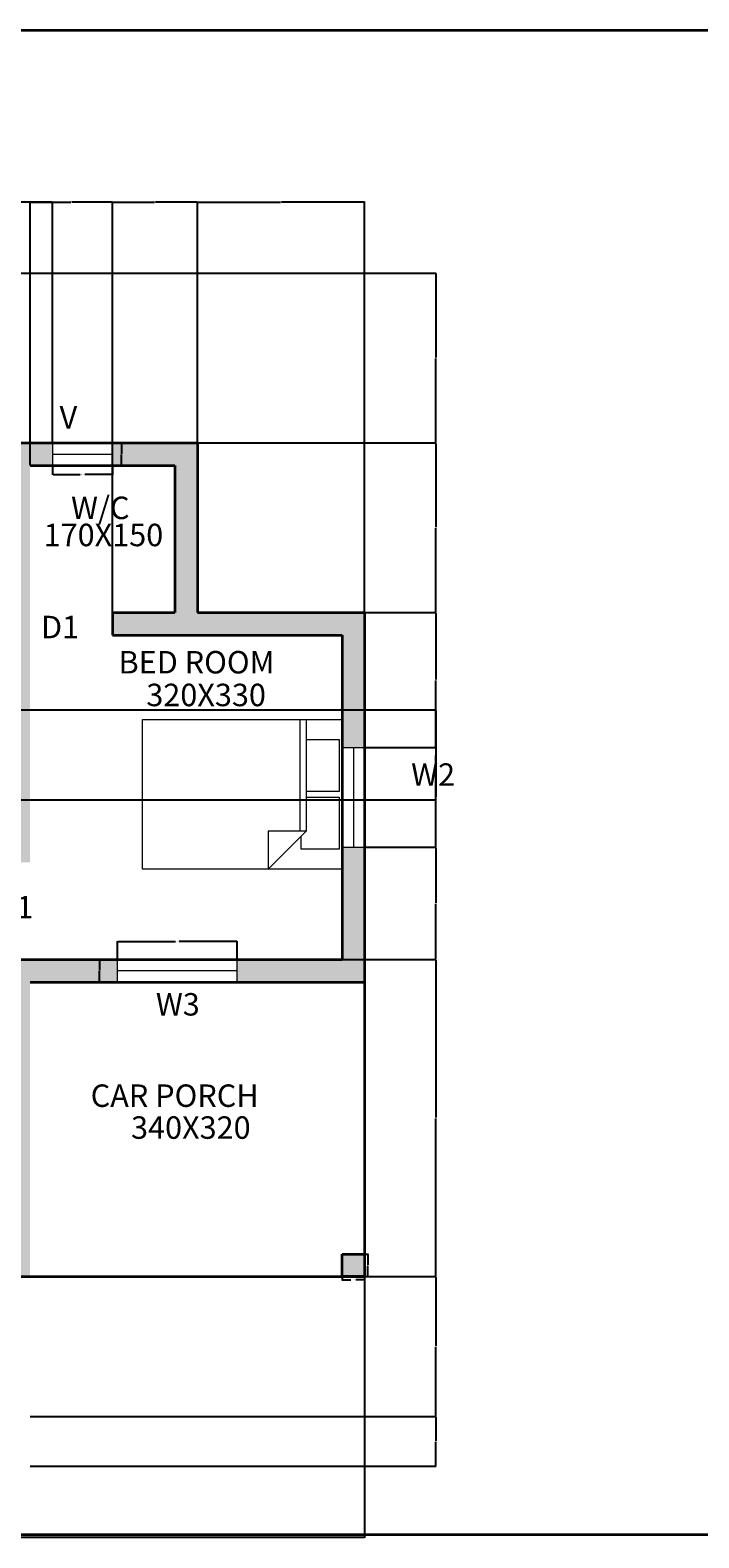
# Model space of a CAD drawing. Units: inches. Extents: x 1332 to 3175, y 1481 to 2088.
# Tile 4 of 5: x 1717 to 1985, y 1484 to 2088. Entities that reach past the tile are written whole.
import ezdxf

# ---------------------------------------------------------------- set-up
doc = ezdxf.new("R2010")
doc.units = ezdxf.units.IN
for name, color, linetype, lineweight in [('A-ANNO-DIMS', 2, 'Continuous', 18), ('A-ANNO-TEXT', 7, 'Continuous', 18), ('A-ANNO-TTLB', 7, 'Continuous', 35), ('A-AREA-IDEN', 7, 'Continuous', 18), ('A-FURN', 8, 'Continuous', 18), ('A-WALL', 7, 'Continuous', 35)]:
    doc.layers.add(name, color=color, linetype=linetype, lineweight=lineweight)
for name, color, linetype, lineweight, true_color in [('A-COLS', 18, 'Continuous', 35, 0x000000), ('A-GLAZ', 30, 'Continuous', 18, 0xf8991e), ('A-WALL-PATT', 18, 'Continuous', 13, 0x000000)]:
    doc.layers.add(name, color=color, linetype=linetype, lineweight=lineweight, true_color=true_color)
doc.styles.get("Standard").update_dxf_attribs({"font": 'arial.ttf'})
doc.dimstyles.get("Standard").update_dxf_attribs({"dimtxt": 0.18, "dimasz": 0.18, "dimexe": 0.18, "dimexo": 0.0625, "dimgap": 0.09, "dimtad": 0, "dimtih": 1, "dimtoh": 1, "dimdec": 4, "dimzin": 0, "dimdsep": 46, "dimtxsty": 'Standard', "dimcen": 0.09, "dimadec": 0, "dimazin": 0, "dimtfac": 1, "dimtdec": 4, "dimtofl": 0, "dimtmove": 0, "dimatfit": 3, "dimfxl": 1, "dimtolj": 1, "dimtzin": 0, "dimarcsym": 0})

# ---------------------------------------------------------------- blocks, each defined once
blk = doc.blocks.new('Bed - Queen')
for p, q in [((0, -80.00003), (0, 0)), ((0, 0), (59.99999, 0)), ((59.99999, 0), (59.99999, -80.00003)), ((7.99999, -1.2), (28.79998, -1.2)), ((7.99999, -14.4), (7.99999, -1.2)), ((28.79998, -1.2), (28.79998, -14.4)), ((31.19999, -1.2), (51.99999, -1.2)), ((31.19999, -14.4), (31.19999, -1.2)), ((51.99999, -1.2), (51.99999, -16.4)), ((0, -14.4), (44.8, -14.4)), ((44.8, -16.8), (0, -16.8)), ((59.99999, -29.6), (44.8, -14.4)), ((44.8, -14.4), (44.8, -29.6)), ((51.99999, -16.4), (46.79936, -16.4)), ((44.8, -29.6), (59.99999, -29.6)), ((59.99999, -80.00003), (0, -80.00003))]:
    blk.add_line(p, q)
blk = doc.blocks.new('COL-SQUARE-9-PLAN')
h = blk.add_hatch(color=256)
h.dxf.hatch_style = 1
h.paths.add_polyline_path([(9, 9), (0, 9), (0, 0), (9, 0)])
blk.add_lwpolyline([(0, 9), (9, 9), (9, 0), (0, 0)], close=True)
blk = doc.blocks.new('WIN-W3-48')
for p, q in [((0, 9), (0, 0)), ((48, 9), (48, 0)), ((0, 4.5), (48, 4.5))]:
    blk.add_line(p, q)
blk = doc.blocks.new('VENT-24')
for p, q in [((0, 9), (0, 0)), ((24, 9), (24, 0)), ((0, 4.5), (24, 4.5))]:
    blk.add_line(p, q)
blk = doc.blocks.new('*D15')
at = {"layer": 'A-ANNO-DIMS', "color": 0, "lineweight": -2, "transparency": 16777216}
for p, q in [((1752.13, 1716.18), (1752.13, 1723.5)), ((1752.31, 1723.32), (1775.38, 1723.32)), ((1799.95, 1723.32), (1776.89, 1723.32)), ((1800.13, 1716.18), (1800.13, 1723.5))]:
    blk.add_line(p, q, dxfattribs=at)
at = {"layer": 'A-ANNO-DIMS', "color": 0, "transparency": 16777216}
for points in [[(1752.31, 1723.35), (1752.31, 1723.29), (1752.13, 1723.32)], [(1799.95, 1723.35), (1799.95, 1723.29), (1800.13, 1723.32)]]:
    blk.add_solid(points, dxfattribs=at)
at = {"layer": 'Defpoints', "color": 0, "transparency": 16777216}
for p in [(1752.13, 1723.32), (1752.13, 1716.12), (1800.13, 1716.12)]:
    blk.add_point(p, dxfattribs=at)
at = {"layer": 'A-ANNO-DIMS', "color": 0, "transparency": 16777216, "insert": (1776.13, 1723.32), "char_height": 0.18, "attachment_point": 5}
blk.add_mtext('\\A1;W3 48 TYP.', dxfattribs=at)
blk = doc.blocks.new('*D16')
at = {"layer": 'A-ANNO-DIMS', "color": 0, "lineweight": -2, "transparency": 16777216}
for p, q in [((1752.07, 1716.12), (1744.75, 1716.12)), ((1744.93, 1715.94), (1744.93, 1711.8)), ((1744.93, 1707.3), (1744.93, 1711.44)), ((1752.07, 1707.12), (1744.75, 1707.12))]:
    blk.add_line(p, q, dxfattribs=at)
at = {"layer": 'A-ANNO-DIMS', "color": 0, "transparency": 16777216}
for points in [[(1744.9, 1715.94), (1744.96, 1715.94), (1744.93, 1716.12)], [(1744.9, 1707.3), (1744.96, 1707.3), (1744.93, 1707.12)]]:
    blk.add_solid(points, dxfattribs=at)
at = {"layer": 'Defpoints', "color": 0, "transparency": 16777216}
for p in [(1752.13, 1716.12), (1744.93, 1707.12), (1752.13, 1707.12)]:
    blk.add_point(p, dxfattribs=at)
at = {"layer": 'A-ANNO-DIMS', "color": 0, "transparency": 16777216, "insert": (1744.93, 1711.62), "char_height": 0.18, "attachment_point": 5}
blk.add_mtext('\\A1;9 TYP.', dxfattribs=at)
blk = doc.blocks.new('*D17')
at = {"layer": 'A-ANNO-DIMS', "color": 0, "lineweight": -2, "transparency": 16777216}
for p, q in [((1726.13, 1914.06), (1726.13, 1910.34)), ((1726.31, 1910.52), (1737.23, 1910.52)), ((1749.95, 1910.52), (1739.03, 1910.52)), ((1750.13, 1914.06), (1750.13, 1910.34))]:
    blk.add_line(p, q, dxfattribs=at)
at = {"layer": 'A-ANNO-DIMS', "color": 0, "transparency": 16777216}
for points in [[(1726.31, 1910.55), (1726.31, 1910.49), (1726.13, 1910.52)], [(1749.95, 1910.55), (1749.95, 1910.49), (1750.13, 1910.52)]]:
    blk.add_solid(points, dxfattribs=at)
at = {"layer": 'Defpoints', "color": 0, "transparency": 16777216}
for p in [(1726.13, 1914.12), (1750.13, 1914.12), (1750.13, 1910.52)]:
    blk.add_point(p, dxfattribs=at)
at = {"layer": 'A-ANNO-DIMS', "color": 0, "transparency": 16777216, "insert": (1738.13, 1910.52), "char_height": 0.18, "attachment_point": 5}
blk.add_mtext('\\A1;VENT 24 TYP.', dxfattribs=at)
blk = doc.blocks.new('*D18')
at = {"layer": 'A-ANNO-DIMS', "color": 0, "lineweight": -2, "transparency": 16777216}
for p, q in [((1750.19, 1923.12), (1753.91, 1923.12)), ((1753.73, 1922.94), (1753.73, 1918.8)), ((1753.73, 1914.3), (1753.73, 1918.44)), ((1750.19, 1914.12), (1753.91, 1914.12))]:
    blk.add_line(p, q, dxfattribs=at)
at = {"layer": 'A-ANNO-DIMS', "color": 0, "transparency": 16777216}
for points in [[(1753.7, 1922.94), (1753.76, 1922.94), (1753.73, 1923.12)], [(1753.7, 1914.3), (1753.76, 1914.3), (1753.73, 1914.12)]]:
    blk.add_solid(points, dxfattribs=at)
at = {"layer": 'Defpoints', "color": 0, "transparency": 16777216}
for p in [(1750.13, 1923.12), (1753.73, 1923.12), (1750.13, 1914.12)]:
    blk.add_point(p, dxfattribs=at)
at = {"layer": 'A-ANNO-DIMS', "color": 0, "transparency": 16777216, "insert": (1753.73, 1918.62), "char_height": 0.18, "attachment_point": 5}
blk.add_mtext('\\A1;9 TYP.', dxfattribs=at)
blk = doc.blocks.new('*D23')
at = {"layer": 'A-ANNO-DIMS', "color": 0, "lineweight": -2, "transparency": 16777216}
for p, q in [((1842.13, 1589.06), (1842.13, 1587.59)), ((1851.13, 1589.06), (1851.13, 1587.59)), ((1842.31, 1587.77), (1845.59, 1587.77)), ((1850.95, 1587.77), (1847.67, 1587.77))]:
    blk.add_line(p, q, dxfattribs=at)
at = {"layer": 'A-ANNO-DIMS', "color": 0, "transparency": 16777216}
for points in [[(1842.31, 1587.8), (1842.31, 1587.74), (1842.13, 1587.77)], [(1850.95, 1587.8), (1850.95, 1587.74), (1851.13, 1587.77)]]:
    blk.add_solid(points, dxfattribs=at)
at = {"layer": 'Defpoints', "color": 0, "transparency": 16777216}
for p in [(1842.13, 1589.12), (1851.13, 1589.12), (1851.13, 1587.77)]:
    blk.add_point(p, dxfattribs=at)
at = {"layer": 'A-ANNO-DIMS', "color": 0, "transparency": 16777216, "insert": (1846.63, 1587.77), "char_height": 0.18, "attachment_point": 5}
blk.add_mtext('\\A1;COLUMN 9 TYP.', dxfattribs=at)
blk = doc.blocks.new('*D24')
at = {"layer": 'A-ANNO-DIMS', "color": 0, "lineweight": -2, "transparency": 16777216}
for p, q in [((1851.19, 1598.12), (1852.66, 1598.12)), ((1852.48, 1597.94), (1852.48, 1593.8)), ((1851.19, 1589.12), (1852.66, 1589.12)), ((1852.48, 1589.3), (1852.48, 1593.44))]:
    blk.add_line(p, q, dxfattribs=at)
at = {"layer": 'A-ANNO-DIMS', "color": 0, "transparency": 16777216}
for points in [[(1852.45, 1597.94), (1852.51, 1597.94), (1852.48, 1598.12)], [(1852.45, 1589.3), (1852.51, 1589.3), (1852.48, 1589.12)]]:
    blk.add_solid(points, dxfattribs=at)
at = {"layer": 'Defpoints', "color": 0, "transparency": 16777216}
for p in [(1851.13, 1598.12), (1852.48, 1598.12), (1851.13, 1589.12)]:
    blk.add_point(p, dxfattribs=at)
at = {"layer": 'A-ANNO-DIMS', "color": 0, "transparency": 16777216, "insert": (1852.48, 1593.62), "char_height": 0.18, "attachment_point": 5}
blk.add_mtext('\\A1;9 TYP.', dxfattribs=at)
blk = doc.blocks.new('*D37')
at = {"layer": 'A-ANNO-DIMS', "color": 0, "lineweight": -2, "transparency": 16777216}
for p, q in [((1851.13, 1589.06), (1851.13, 1484.44)), ((1389.63, 1533.06), (1389.63, 1484.44)), ((1389.81, 1484.62), (1619.98, 1484.62)), ((1850.95, 1484.62), (1620.78, 1484.62))]:
    blk.add_line(p, q, dxfattribs=at)
at = {"layer": 'A-ANNO-DIMS', "color": 0, "transparency": 16777216}
for points in [[(1389.81, 1484.65), (1389.81, 1484.59), (1389.63, 1484.62)], [(1850.95, 1484.65), (1850.95, 1484.59), (1851.13, 1484.62)]]:
    blk.add_solid(points, dxfattribs=at)
at = {"layer": 'Defpoints', "color": 0, "transparency": 16777216}
for p in [(1851.13, 1589.12), (1389.63, 1533.12), (1851.13, 1484.62)]:
    blk.add_point(p, dxfattribs=at)
at = {"layer": 'A-ANNO-DIMS', "color": 0, "transparency": 16777216, "insert": (1620.38, 1484.62), "char_height": 0.18, "attachment_point": 5}
blk.add_mtext('\\A1;461.5', dxfattribs=at)
blk = doc.blocks.new('*D45')
at = {"layer": 'A-ANNO-DIMS', "color": 0, "lineweight": -2, "transparency": 16777216}
for p, q in [((1673.13, 1923.18), (1673.13, 2019.8)), ((1673.31, 2019.62), (1699.41, 2019.62)), ((1725.95, 2019.62), (1699.85, 2019.62)), ((1726.13, 1923.18), (1726.13, 2019.8))]:
    blk.add_line(p, q, dxfattribs=at)
at = {"layer": 'A-ANNO-DIMS', "color": 0, "transparency": 16777216}
for points in [[(1673.31, 2019.65), (1673.31, 2019.59), (1673.13, 2019.62)], [(1725.95, 2019.65), (1725.95, 2019.59), (1726.13, 2019.62)]]:
    blk.add_solid(points, dxfattribs=at)
at = {"layer": 'Defpoints', "color": 0, "transparency": 16777216}
for p in [(1726.13, 2019.62), (1673.13, 1923.12), (1726.13, 1923.12)]:
    blk.add_point(p, dxfattribs=at)
at = {"layer": 'A-ANNO-DIMS', "color": 0, "transparency": 16777216, "insert": (1699.63, 2019.62), "char_height": 0.18, "attachment_point": 5}
blk.add_mtext('\\A1;53', dxfattribs=at)
blk = doc.blocks.new('*D46')
at = {"layer": 'A-ANNO-DIMS', "color": 0, "lineweight": -2, "transparency": 16777216}
for p, q in [((1750.13, 1923.18), (1750.13, 2019.8)), ((1750.31, 2019.62), (1766.91, 2019.62)), ((1783.95, 2019.62), (1767.35, 2019.62)), ((1784.13, 1923.18), (1784.13, 2019.8))]:
    blk.add_line(p, q, dxfattribs=at)
at = {"layer": 'A-ANNO-DIMS', "color": 0, "transparency": 16777216}
for points in [[(1750.31, 2019.65), (1750.31, 2019.59), (1750.13, 2019.62)], [(1783.95, 2019.65), (1783.95, 2019.59), (1784.13, 2019.62)]]:
    blk.add_solid(points, dxfattribs=at)
at = {"layer": 'Defpoints', "color": 0, "transparency": 16777216}
for p in [(1784.13, 2019.62), (1750.13, 1923.12), (1784.13, 1923.12)]:
    blk.add_point(p, dxfattribs=at)
at = {"layer": 'A-ANNO-DIMS', "color": 0, "transparency": 16777216, "insert": (1767.13, 2019.62), "char_height": 0.18, "attachment_point": 5}
blk.add_mtext('\\A1;34', dxfattribs=at)
blk = doc.blocks.new('*D47')
at = {"layer": 'A-ANNO-DIMS', "color": 0, "lineweight": -2, "transparency": 16777216}
for p, q in [((1784.13, 1923.18), (1784.13, 2019.8)), ((1784.31, 2019.62), (1817.41, 2019.62)), ((1850.95, 2019.62), (1817.85, 2019.62)), ((1851.13, 1855.18), (1851.13, 2019.8))]:
    blk.add_line(p, q, dxfattribs=at)
at = {"layer": 'A-ANNO-DIMS', "color": 0, "transparency": 16777216}
for points in [[(1784.31, 2019.65), (1784.31, 2019.59), (1784.13, 2019.62)], [(1850.95, 2019.65), (1850.95, 2019.59), (1851.13, 2019.62)]]:
    blk.add_solid(points, dxfattribs=at)
at = {"layer": 'Defpoints', "color": 0, "transparency": 16777216}
for p in [(1851.13, 2019.62), (1784.13, 1923.12), (1851.13, 1855.12)]:
    blk.add_point(p, dxfattribs=at)
at = {"layer": 'A-ANNO-DIMS', "color": 0, "transparency": 16777216, "insert": (1817.63, 2019.62), "char_height": 0.18, "attachment_point": 5}
blk.add_mtext('\\A1;67', dxfattribs=at)
blk = doc.blocks.new('*D48')
at = {"layer": 'A-ANNO-DIMS', "color": 0, "lineweight": -2, "transparency": 16777216}
for p, q in [((1717.19, 1533.12), (1879.81, 1533.12)), ((1879.63, 1532.94), (1879.63, 1523.3)), ((1879.63, 1513.3), (1879.63, 1522.94)), ((1717.19, 1513.12), (1879.81, 1513.12))]:
    blk.add_line(p, q, dxfattribs=at)
at = {"layer": 'A-ANNO-DIMS', "color": 0, "transparency": 16777216}
for points in [[(1879.6, 1532.94), (1879.66, 1532.94), (1879.63, 1533.12)], [(1879.6, 1513.3), (1879.66, 1513.3), (1879.63, 1513.12)]]:
    blk.add_solid(points, dxfattribs=at)
at = {"layer": 'Defpoints', "color": 0, "transparency": 16777216}
for p in [(1717.13, 1533.12), (1879.63, 1533.12), (1717.13, 1513.12)]:
    blk.add_point(p, dxfattribs=at)
at = {"layer": 'A-ANNO-DIMS', "color": 0, "transparency": 16777216, "insert": (1879.63, 1523.12), "char_height": 0.18, "attachment_point": 5}
blk.add_mtext('\\A1;20', dxfattribs=at)
blk = doc.blocks.new('*D49')
at = {"layer": 'A-ANNO-DIMS', "color": 0, "lineweight": -2, "transparency": 16777216}
for p, q in [((1851.19, 1589.12), (1879.81, 1589.12)), ((1879.63, 1588.94), (1879.63, 1561.3)), ((1879.63, 1533.3), (1879.63, 1560.94)), ((1717.19, 1533.12), (1879.81, 1533.12))]:
    blk.add_line(p, q, dxfattribs=at)
at = {"layer": 'A-ANNO-DIMS', "color": 0, "transparency": 16777216}
for points in [[(1879.6, 1588.94), (1879.66, 1588.94), (1879.63, 1589.12)], [(1879.6, 1533.3), (1879.66, 1533.3), (1879.63, 1533.12)]]:
    blk.add_solid(points, dxfattribs=at)
at = {"layer": 'Defpoints', "color": 0, "transparency": 16777216}
for p in [(1851.13, 1589.12), (1879.63, 1589.12), (1717.13, 1533.12)]:
    blk.add_point(p, dxfattribs=at)
at = {"layer": 'A-ANNO-DIMS', "color": 0, "transparency": 16777216, "insert": (1879.63, 1561.12), "char_height": 0.18, "attachment_point": 5}
blk.add_mtext('\\A1;56', dxfattribs=at)
blk = doc.blocks.new('*D50')
at = {"layer": 'A-ANNO-DIMS', "color": 0, "lineweight": -2, "transparency": 16777216}
for p, q in [((1842.19, 1716.12), (1879.81, 1716.12)), ((1879.63, 1715.94), (1879.63, 1652.8)), ((1879.63, 1589.3), (1879.63, 1652.44)), ((1851.19, 1589.12), (1879.81, 1589.12))]:
    blk.add_line(p, q, dxfattribs=at)
at = {"layer": 'A-ANNO-DIMS', "color": 0, "transparency": 16777216}
for points in [[(1879.6, 1715.94), (1879.66, 1715.94), (1879.63, 1716.12)], [(1879.6, 1589.3), (1879.66, 1589.3), (1879.63, 1589.12)]]:
    blk.add_solid(points, dxfattribs=at)
at = {"layer": 'Defpoints', "color": 0, "transparency": 16777216}
for p in [(1842.13, 1716.12), (1879.63, 1716.12), (1851.13, 1589.12)]:
    blk.add_point(p, dxfattribs=at)
at = {"layer": 'A-ANNO-DIMS', "color": 0, "transparency": 16777216, "insert": (1879.63, 1652.62), "char_height": 0.18, "attachment_point": 5}
blk.add_mtext('\\A1;127', dxfattribs=at)
blk = doc.blocks.new('*D51')
at = {"layer": 'A-ANNO-DIMS', "color": 0, "lineweight": -2, "transparency": 16777216}
for p, q in [((1851.19, 1761.12), (1879.81, 1761.12)), ((1879.63, 1760.94), (1879.63, 1738.8)), ((1879.63, 1716.3), (1879.63, 1738.44)), ((1842.19, 1716.12), (1879.81, 1716.12))]:
    blk.add_line(p, q, dxfattribs=at)
at = {"layer": 'A-ANNO-DIMS', "color": 0, "transparency": 16777216}
for points in [[(1879.6, 1760.94), (1879.66, 1760.94), (1879.63, 1761.12)], [(1879.6, 1716.3), (1879.66, 1716.3), (1879.63, 1716.12)]]:
    blk.add_solid(points, dxfattribs=at)
at = {"layer": 'Defpoints', "color": 0, "transparency": 16777216}
for p in [(1851.13, 1761.12), (1879.63, 1761.12), (1842.13, 1716.12)]:
    blk.add_point(p, dxfattribs=at)
at = {"layer": 'A-ANNO-DIMS', "color": 0, "transparency": 16777216, "insert": (1879.63, 1738.62), "char_height": 0.18, "attachment_point": 5}
blk.add_mtext('\\A1;45', dxfattribs=at)
blk = doc.blocks.new('*D52')
at = {"layer": 'A-ANNO-DIMS', "color": 0, "lineweight": -2, "transparency": 16777216}
for p, q in [((1851.19, 1801.12), (1879.81, 1801.12)), ((1879.63, 1800.94), (1879.63, 1781.3)), ((1879.63, 1761.3), (1879.63, 1780.94)), ((1851.19, 1761.12), (1879.81, 1761.12))]:
    blk.add_line(p, q, dxfattribs=at)
at = {"layer": 'A-ANNO-DIMS', "color": 0, "transparency": 16777216}
for points in [[(1879.6, 1800.94), (1879.66, 1800.94), (1879.63, 1801.12)], [(1879.6, 1761.3), (1879.66, 1761.3), (1879.63, 1761.12)]]:
    blk.add_solid(points, dxfattribs=at)
at = {"layer": 'Defpoints', "color": 0, "transparency": 16777216}
for p in [(1851.13, 1801.12), (1879.63, 1801.12), (1851.13, 1761.12)]:
    blk.add_point(p, dxfattribs=at)
at = {"layer": 'A-ANNO-DIMS', "color": 0, "transparency": 16777216, "insert": (1879.63, 1781.12), "char_height": 0.18, "attachment_point": 5}
blk.add_mtext('\\A1;40', dxfattribs=at)
blk = doc.blocks.new('*D53')
at = {"layer": 'A-ANNO-DIMS', "color": 0, "lineweight": -2, "transparency": 16777216}
for p, q in [((1851.19, 1855.12), (1879.81, 1855.12)), ((1879.63, 1854.94), (1879.63, 1828.3)), ((1879.63, 1801.3), (1879.63, 1827.94)), ((1851.19, 1801.12), (1879.81, 1801.12))]:
    blk.add_line(p, q, dxfattribs=at)
at = {"layer": 'A-ANNO-DIMS', "color": 0, "transparency": 16777216}
for points in [[(1879.6, 1854.94), (1879.66, 1854.94), (1879.63, 1855.12)], [(1879.6, 1801.3), (1879.66, 1801.3), (1879.63, 1801.12)]]:
    blk.add_solid(points, dxfattribs=at)
at = {"layer": 'Defpoints', "color": 0, "transparency": 16777216}
for p in [(1851.13, 1855.12), (1879.63, 1855.12), (1851.13, 1801.12)]:
    blk.add_point(p, dxfattribs=at)
at = {"layer": 'A-ANNO-DIMS', "color": 0, "transparency": 16777216, "insert": (1879.63, 1828.12), "char_height": 0.18, "attachment_point": 5}
blk.add_mtext('\\A1;54', dxfattribs=at)
blk = doc.blocks.new('*D54')
at = {"layer": 'A-ANNO-DIMS', "color": 0, "lineweight": -2, "transparency": 16777216}
for p, q in [((1784.19, 1923.12), (1879.81, 1923.12)), ((1879.63, 1922.94), (1879.63, 1889.3)), ((1879.63, 1855.3), (1879.63, 1888.94)), ((1851.19, 1855.12), (1879.81, 1855.12))]:
    blk.add_line(p, q, dxfattribs=at)
at = {"layer": 'A-ANNO-DIMS', "color": 0, "transparency": 16777216}
for points in [[(1879.6, 1922.94), (1879.66, 1922.94), (1879.63, 1923.12)], [(1879.6, 1855.3), (1879.66, 1855.3), (1879.63, 1855.12)]]:
    blk.add_solid(points, dxfattribs=at)
at = {"layer": 'Defpoints', "color": 0, "transparency": 16777216}
for p in [(1784.13, 1923.12), (1879.63, 1923.12), (1851.13, 1855.12)]:
    blk.add_point(p, dxfattribs=at)
at = {"layer": 'A-ANNO-DIMS', "color": 0, "transparency": 16777216, "insert": (1879.63, 1889.12), "char_height": 0.18, "attachment_point": 5}
blk.add_mtext('\\A1;68', dxfattribs=at)
blk = doc.blocks.new('*D55')
at = {"layer": 'A-ANNO-DIMS', "color": 0, "lineweight": -2, "transparency": 16777216}
for p, q in [((1541.69, 1991.12), (1879.81, 1991.12)), ((1879.63, 1990.94), (1879.63, 1957.3)), ((1879.63, 1923.3), (1879.63, 1956.94)), ((1784.19, 1923.12), (1879.81, 1923.12))]:
    blk.add_line(p, q, dxfattribs=at)
at = {"layer": 'A-ANNO-DIMS', "color": 0, "transparency": 16777216}
for points in [[(1879.6, 1990.94), (1879.66, 1990.94), (1879.63, 1991.12)], [(1879.6, 1923.3), (1879.66, 1923.3), (1879.63, 1923.12)]]:
    blk.add_solid(points, dxfattribs=at)
at = {"layer": 'Defpoints', "color": 0, "transparency": 16777216}
for p in [(1541.63, 1991.12), (1879.63, 1991.12), (1784.13, 1923.12)]:
    blk.add_point(p, dxfattribs=at)
at = {"layer": 'A-ANNO-DIMS', "color": 0, "transparency": 16777216, "insert": (1879.63, 1957.12), "char_height": 0.18, "attachment_point": 5}
blk.add_mtext('\\A1;68', dxfattribs=at)
blk = doc.blocks.new('*D85')
at = {"layer": 'A-ANNO-DIMS', "color": 0, "lineweight": -2, "transparency": 16777216}
for p, q in [((1717.13, 1914.18), (1717.13, 2019.8)), ((1717.31, 2019.62), (1733.41, 2019.62)), ((1749.95, 2019.62), (1733.85, 2019.62)), ((1750.13, 1855.18), (1750.13, 2019.8))]:
    blk.add_line(p, q, dxfattribs=at)
at = {"layer": 'A-ANNO-DIMS', "color": 0, "transparency": 16777216}
for points in [[(1717.31, 2019.65), (1717.31, 2019.59), (1717.13, 2019.62)], [(1749.95, 2019.65), (1749.95, 2019.59), (1750.13, 2019.62)]]:
    blk.add_solid(points, dxfattribs=at)
at = {"layer": 'Defpoints', "color": 0, "transparency": 16777216}
for p in [(1750.13, 2019.62), (1717.13, 1914.12), (1750.13, 1855.12)]:
    blk.add_point(p, dxfattribs=at)
at = {"layer": 'A-ANNO-DIMS', "color": 0, "transparency": 16777216, "insert": (1733.63, 2019.62), "char_height": 0.18, "attachment_point": 5}
blk.add_mtext('\\A1;33', dxfattribs=at)
blk = doc.blocks.new('*D88')
at = {"layer": 'A-ANNO-DIMS', "color": 0, "lineweight": -2, "transparency": 16777216}
for p, q in [((1532.69, 1816.12), (1879.81, 1816.12)), ((1879.63, 1815.94), (1879.63, 1798.3)), ((1879.63, 1780.3), (1879.63, 1797.94)), ((1532.69, 1780.12), (1879.81, 1780.12))]:
    blk.add_line(p, q, dxfattribs=at)
at = {"layer": 'A-ANNO-DIMS', "color": 0, "transparency": 16777216}
for points in [[(1879.6, 1815.94), (1879.66, 1815.94), (1879.63, 1816.12)], [(1879.6, 1780.3), (1879.66, 1780.3), (1879.63, 1780.12)]]:
    blk.add_solid(points, dxfattribs=at)
at = {"layer": 'Defpoints', "color": 0, "transparency": 16777216}
for p in [(1532.63, 1816.12), (1879.63, 1816.12), (1532.63, 1780.12)]:
    blk.add_point(p, dxfattribs=at)
at = {"layer": 'A-ANNO-DIMS', "color": 0, "transparency": 16777216, "insert": (1879.63, 1798.12), "char_height": 0.18, "attachment_point": 5}
blk.add_mtext('\\A1;36', dxfattribs=at)

msp = doc.modelspace()

# ---------------------------------------------------------------- hatches: boundary and pattern name
at = {"layer": 'A-WALL-PATT'}
h = msp.add_hatch(color=256, dxfattribs=at)
h.dxf.hatch_style = 1
h.paths.add_polyline_path([(1398.6316, 1914.1183), (1442.6316, 1914.1183), (1442.6316, 1923.1183), (1389.6316, 1923.1183), (1389.6316, 1868.1183), (1398.6316, 1868.1183)])
h.paths.add_polyline_path([(1398.6316, 1828.1183), (1389.6316, 1828.1183), (1389.6316, 1759.1183), (1398.6316, 1759.1183), (1398.6316, 1771.1183), (1477.6316, 1771.1183), (1477.6316, 1716.1183), (1437.6316, 1716.1183), (1437.6316, 1707.1183), (1493.6316, 1707.1183), (1493.6316, 1716.1183), (1486.6316, 1716.1183), (1486.6316, 1771.1183), (1532.6316, 1771.1183), (1532.6316, 1780.1183), (1398.6316, 1780.1183)])
h.paths.add_polyline_path([(1398.6316, 1735.1183), (1389.6316, 1735.1183), (1389.6316, 1647.6183), (1398.6316, 1647.6183)])
h.paths.add_polyline_path([(1398.6316, 1599.6183), (1389.6316, 1599.6183), (1389.6316, 1533.1183), (1442.6316, 1533.1183), (1442.6316, 1542.1183), (1398.6316, 1542.1183)])
h.paths.add_polyline_path([(1541.6316, 1589.1183), (1576.5616, 1589.1183), (1576.5616, 1598.1183), (1541.6316, 1598.1183), (1541.6316, 1707.1183), (1576.5616, 1707.1183), (1576.5616, 1716.1183), (1532.6316, 1716.1183), (1532.6316, 1542.1183), (1490.6316, 1542.1183), (1490.6316, 1533.1183), (1541.6316, 1533.1183)])
h.paths.add_polyline_path([(1717.1316, 1707.1183), (1752.1316, 1707.1183), (1752.1316, 1716.1183), (1672.5616, 1716.1183), (1672.5616, 1707.1183), (1708.1316, 1707.1183), (1708.1316, 1598.1183), (1672.5616, 1598.1183), (1672.5616, 1589.1183), (1717.1316, 1589.1183)])
h.paths.add_polyline_path([(1851.1316, 1761.1183), (1842.1316, 1761.1183), (1842.1316, 1716.1183), (1800.1316, 1716.1183), (1800.1316, 1707.1183), (1851.1316, 1707.1183)])
h.paths.add_polyline_path([(1851.1316, 1855.1183), (1784.1316, 1855.1183), (1784.1316, 1923.1183), (1750.1316, 1923.1183), (1750.1316, 1914.1183), (1775.1316, 1914.1183), (1775.1316, 1855.1183), (1750.1316, 1855.1183), (1750.1316, 1846.1183), (1842.1316, 1846.1183), (1842.1316, 1801.1183), (1851.1316, 1801.1183)])
h.paths.add_polyline_path([(1717.1316, 1914.1183), (1726.1316, 1914.1183), (1726.1316, 1923.1183), (1673.1316, 1923.1183), (1673.1316, 1914.1183), (1708.1316, 1914.1183), (1708.1316, 1755.1183), (1717.1316, 1755.1183)])
h.paths.add_polyline_path([(1661.1316, 1855.1183), (1636.1316, 1855.1183), (1636.1316, 1914.1183), (1649.1316, 1914.1183), (1649.1316, 1923.1183), (1611.3665, 1923.1183), (1611.3665, 1914.1183), (1627.1316, 1914.1183), (1627.1316, 1846.1183), (1661.1316, 1846.1183)])
h.paths.add_polyline_path([(1541.6316, 1914.1183), (1563.3665, 1914.1183), (1563.3665, 1923.1183), (1541.6316, 1923.1183), (1541.6316, 1991.1183), (1528.6316, 1991.1183), (1528.6316, 1982.1183), (1532.6316, 1982.1183), (1532.6316, 1914.1183), (1532.6316, 1816.1183), (1541.6316, 1816.1183)])
h.paths.add_polyline_path([(1453.6316, 1982.1183), (1457.6316, 1982.1183), (1457.6316, 1991.1183), (1444.6316, 1991.1183), (1444.6316, 1956.1183), (1453.6316, 1956.1183)])

# ---------------------------------------------------------------- linework, layer by layer
at = {"layer": 'A-ANNO-TTLB'}
msp.add_lwpolyline([(1332.1674, 2088.4777), (3159.6908, 2088.4777), (3159.6908, 1485.6439), (1332.1674, 1485.6439)], close=True, dxfattribs=at)
at = {"layer": 'A-GLAZ'}
for p, q in [((1842.1316, 1801.1183), (1851.1316, 1801.1183)), ((1846.6316, 1801.1183), (1846.6316, 1761.1183)), ((1842.1316, 1761.1183), (1851.1316, 1761.1183))]:
    msp.add_line(p, q, dxfattribs=at)
at = {"layer": 'A-WALL'}
for p, q in [((1541.6316, 1923.1183), (1784.1316, 1923.1183)), ((1784.1316, 1923.1183), (1784.1316, 1855.1183)), ((1717.1316, 1914.1183), (1775.1316, 1914.1183)), ((1775.1316, 1914.1183), (1775.1316, 1855.1183)), ((1750.1316, 1855.1183), (1775.1316, 1855.1183)), ((1750.1316, 1855.1183), (1750.1316, 1846.1183)), ((1784.1316, 1855.1183), (1851.1316, 1855.1183)), ((1851.1316, 1855.1183), (1851.1316, 1589.1183)), ((1750.1316, 1846.1183), (1842.1316, 1846.1183)), ((1842.1316, 1846.1183), (1842.1316, 1716.1183)), ((1672.5616, 1716.1183), (1842.1316, 1716.1183)), ((1717.1316, 1707.1183), (1851.1316, 1707.1183)), ((1648.5616, 1589.1183), (1851.1316, 1589.1183))]:
    msp.add_line(p, q, dxfattribs=at)

# ---------------------------------------------------------------- block references
at = {"layer": 'A-COLS'}
msp.add_blockref('COL-SQUARE-9-PLAN', (1842.1316, 1589.1183), dxfattribs=at)
at = {"layer": 'A-FURN', "rotation": 270}
msp.add_blockref('Bed - Queen', (1842.1316, 1812.3182), dxfattribs=at)
at = {"layer": 'A-GLAZ'}
msp.add_blockref('VENT-24', (1726.1316, 1914.1183), dxfattribs=at)
at = {"layer": 'A-GLAZ', "rotation": 180}
msp.add_blockref('WIN-W3-48', (1800.1316, 1716.1183), dxfattribs=at)

# ---------------------------------------------------------------- texts
at = {"layer": 'A-ANNO-TEXT'}
for s, p in [('      V', (1712.4208, 1928.8639)), ('      D1', (1704.9881, 1844.8373)), ('    W2', (1858.7841, 1785.7447)), ('      D1', (1686.663, 1732.5865)), ('    W3', (1756.502, 1693.6834))]:
    msp.add_text(s, height=9, dxfattribs=at).set_placement(p)
at = {"layer": 'A-AREA-IDEN'}
for s, p in [('    W/C', (1722.5241, 1892.5929)), ('170X150', (1722.5241, 1881.7283)), (' BED ROOM', (1749.8034, 1830.7461)), ('320X330', (1763.6686, 1817.6349)), ('    CAR PORCH', (1730.3797, 1657.0881)), ('340X320', (1757.5505, 1644.3116))]:
    msp.add_text(s, height=9, dxfattribs=at).set_placement(p)

# ---------------------------------------------------------------- dimensions: what is measured, and where the dimension line sits
at = {"layer": 'A-ANNO-DIMS'}
for base, p1, p2, override, picture, middle in [((1726.1316, 2019.6183), (1673.1316, 1923.1183), (1726.1316, 1923.1183), {"dimdec": 0, "dimlfac": 1, "dimrnd": 0, "dimzin": 0, "dimdsep": 46, "dimlunit": 2}, '*D45', (1699.6316, 2019.6183)), ((1750.1316, 2019.6183), (1717.1316, 1914.1183), (1750.1316, 1855.1183), {"dimdec": 0, "dimlfac": 1, "dimrnd": 0, "dimzin": 0, "dimdsep": 46, "dimlunit": 2}, '*D85', (1733.6316, 2019.6183)), ((1784.1316, 2019.6183), (1750.1316, 1923.1183), (1784.1316, 1923.1183), {"dimdec": 0, "dimlfac": 1, "dimrnd": 0, "dimzin": 0, "dimdsep": 46, "dimlunit": 2}, '*D46', (1767.1316, 2019.6183)), ((1851.1316, 2019.6183), (1784.1316, 1923.1183), (1851.1316, 1855.1183), {"dimdec": 0, "dimlfac": 1, "dimrnd": 0, "dimzin": 0, "dimdsep": 46, "dimlunit": 2}, '*D47', (1817.6316, 2019.6183)), ((1851.1316, 1484.6183), (1389.6316, 1533.1183), (1851.1316, 1589.1183), {"dimdec": 1, "dimlfac": 1, "dimrnd": 0, "dimzin": 0, "dimdsep": 46, "dimlunit": 2}, '*D37', (1620.3816, 1484.6183))]:
    dim = msp.add_linear_dim(base=base, p1=p1, p2=p2, dimstyle='Standard', override=override, dxfattribs=at)
    dim.commit()
    dim.dimension.update_dxf_attribs({"geometry": picture, "text_midpoint": middle})
for base, p1, p2, picture, middle in [((1879.6316, 1991.1183), (1784.1316, 1923.1183), (1541.6316, 1991.1183), '*D55', (1879.6316, 1957.1183)), ((1879.6316, 1923.1183), (1851.1316, 1855.1183), (1784.1316, 1923.1183), '*D54', (1879.6316, 1889.1183)), ((1879.6316, 1855.1183), (1851.1316, 1801.1183), (1851.1316, 1855.1183), '*D53', (1879.6316, 1828.1183)), ((1879.6316, 1816.1183), (1532.6316, 1780.1183), (1532.6316, 1816.1183), '*D88', (1879.6316, 1798.1183)), ((1879.6316, 1801.1183), (1851.1316, 1761.1183), (1851.1316, 1801.1183), '*D52', (1879.6316, 1781.1183)), ((1879.6316, 1761.1183), (1842.1316, 1716.1183), (1851.1316, 1761.1183), '*D51', (1879.6316, 1738.6183)), ((1879.6316, 1716.1183), (1851.1316, 1589.1183), (1842.1316, 1716.1183), '*D50', (1879.6316, 1652.6183)), ((1879.6316, 1589.1183), (1717.1316, 1533.1183), (1851.1316, 1589.1183), '*D49', (1879.6316, 1561.1183)), ((1879.6316, 1533.1183), (1717.1316, 1513.1183), (1717.1316, 1533.1183), '*D48', (1879.6316, 1523.1183))]:
    dim = msp.add_linear_dim(base=base, p1=p1, p2=p2, angle=90, dimstyle='Standard', override={"dimdec": 0, "dimlfac": 1, "dimrnd": 0, "dimzin": 0, "dimdsep": 46, "dimlunit": 2}, dxfattribs=at)
    dim.commit()
    dim.dimension.update_dxf_attribs({"geometry": picture, "text_midpoint": middle})
for base, p1, p2, angle, text, picture, middle in [((1753.7316, 1923.1183), (1750.1316, 1914.1183), (1750.1316, 1923.1183), 90, '<> TYP.', '*D18', (1753.7316, 1918.6183)), ((1752.1316, 1723.3183), (1800.1316, 1716.1183), (1752.1316, 1716.1183), 180, 'W3 <> TYP.', '*D15', (1776.1316, 1723.3183)), ((1744.9316, 1707.1183), (1752.1316, 1716.1183), (1752.1316, 1707.1183), 270, '<> TYP.', '*D16', (1744.9316, 1711.6183)), ((1852.4816, 1598.1183), (1851.1316, 1589.1183), (1851.1316, 1598.1183), 90, '<> TYP.', '*D24', (1852.4816, 1593.6183))]:
    dim = msp.add_linear_dim(base=base, p1=p1, p2=p2, angle=angle, text=text, dimstyle='Standard', override={"dimdec": 0, "dimlfac": 1, "dimrnd": 0, "dimzin": 0, "dimdsep": 46, "dimlunit": 2}, dxfattribs=at)
    dim.commit()
    dim.dimension.update_dxf_attribs({"geometry": picture, "text_midpoint": middle})
for base, p1, p2, text, picture, middle in [((1750.1316, 1910.5183), (1726.1316, 1914.1183), (1750.1316, 1914.1183), 'VENT <> TYP.', '*D17', (1738.1316, 1910.5183)), ((1851.1316, 1587.7683), (1842.1316, 1589.1183), (1851.1316, 1589.1183), 'COLUMN <> TYP.', '*D23', (1846.6316, 1587.7683))]:
    dim = msp.add_linear_dim(base=base, p1=p1, p2=p2, text=text, dimstyle='Standard', override={"dimdec": 0, "dimlfac": 1, "dimrnd": 0, "dimzin": 0, "dimdsep": 46, "dimlunit": 2}, dxfattribs=at)
    dim.commit()
    dim.dimension.update_dxf_attribs({"geometry": picture, "text_midpoint": middle})

doc.saveas('drawing.dxf')
